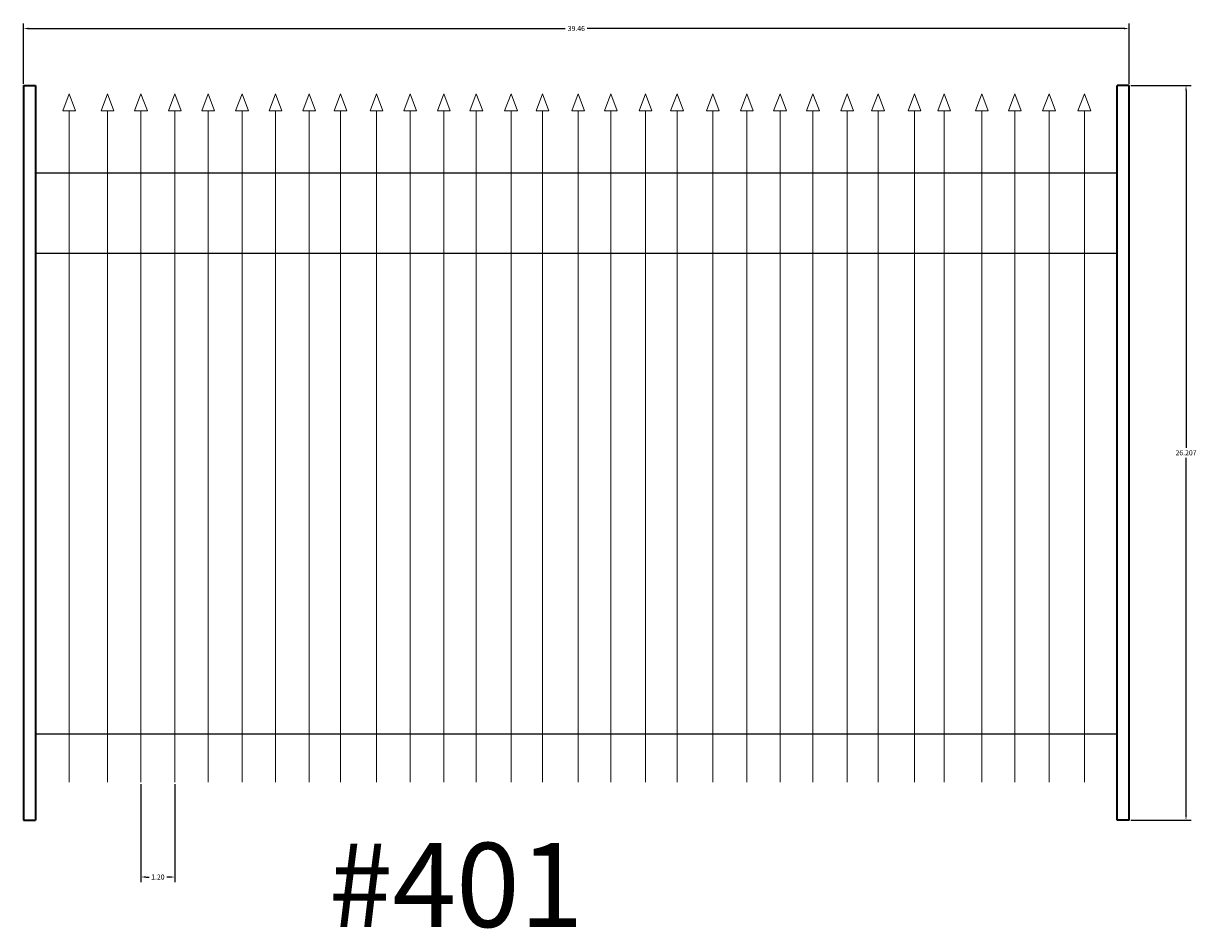
# Model space of a CAD drawing. Units: inches. Extents: x 756 to 915, y 488 to 695.
# Tile 23 of 25: x 866 to 908, y 626 to 659. Entities that reach past the tile are written whole.
import ezdxf

# ---------------------------------------------------------------- set-up
doc = ezdxf.new("R2010")
doc.units = ezdxf.units.IN
doc.header["$MEASUREMENT"] = 0
for name, color, linetype, lineweight in [('L-ANNO-TEXT', 7, 'Continuous', 25), ('L-FENC-PCKT', 7, 'Continuous', 18), ('L-FENC-POST', 7, 'Continuous', 35), ('L-FENC-RAIL', 7, 'Continuous', 25), ('M-DIMS', 2, 'Continuous', 18)]:
    doc.layers.add(name, color=color, linetype=linetype, lineweight=lineweight)
doc.styles.get("Standard").update_dxf_attribs({"font": 'arial.ttf'})
doc.dimstyles.get("Standard").update_dxf_attribs({"dimtxt": 0.18, "dimasz": 0.18, "dimexe": 0.18, "dimexo": 0.0625, "dimgap": 0.09, "dimtad": 0, "dimtih": 1, "dimtoh": 1, "dimdec": 0, "dimzin": 0, "dimdsep": 46, "dimlunit": 3, "dimtxsty": 'Standard', "dimcen": 0.09, "dimadec": 0, "dimazin": 0, "dimtfac": 1, "dimtdec": 0, "dimtofl": 0, "dimtmove": 0, "dimatfit": 3, "dimfxl": 1, "dimtolj": 1, "dimtzin": 0, "dimarcsym": 0})

# ---------------------------------------------------------------- blocks, each defined once
blk = doc.blocks.new('PICKET-SPEAR-EXTENDED')
blk.add_line((0.228, 23.946), (0.228, 0))
blk.add_lwpolyline([(0.228, 23.946), (0, 23.946), (0.228, 24.558), (0.455, 23.946)], close=True)
blk = doc.blocks.new('FENCE-POST-LEFT')
for p, q in [((0, 26.207), (0, 0)), ((0, 26.207), (0.426, 26.207)), ((0.426, 26.207), (0.426, 0)), ((0.426, 26.207), (0.426, 0)), ((0, 0), (0.426, 0))]:
    blk.add_line(p, q)
blk = doc.blocks.new('FENCE-POST-RIGHT')
for p, q in [((0, 26.207), (0, 0)), ((0, 26.207), (0.427, 26.207)), ((0.427, 26.207), (0.427, 0)), ((0, 0), (0.427, 0))]:
    blk.add_line(p, q)
blk = doc.blocks.new('*D41')
at = {"layer": 'Defpoints', "color": 0, "transparency": 16777216}
for p in [(905.412, 658.397), (865.954, 656.367), (905.412, 656.367)]:
    blk.add_point(p, dxfattribs=at)
at = {"layer": 'M-DIMS', "color": 0, "lineweight": -2, "transparency": 16777216}
for p, q in [((865.954, 656.429), (865.954, 658.577)), ((905.412, 656.429), (905.412, 658.577)), ((866.134, 658.397), (885.289, 658.397)), ((905.232, 658.397), (886.076, 658.397))]:
    blk.add_line(p, q, dxfattribs=at)
at = {"layer": 'M-DIMS', "color": 0, "transparency": 16777216}
for points in [[(866.134, 658.427), (866.134, 658.367), (865.954, 658.397)], [(905.232, 658.427), (905.232, 658.367), (905.412, 658.397)]]:
    blk.add_solid(points, dxfattribs=at)
at = {"layer": 'M-DIMS', "color": 0, "transparency": 16777216, "insert": (885.683, 658.397), "char_height": 0.18, "attachment_point": 5}
blk.add_mtext('\\A1;39.46', dxfattribs=at)
blk = doc.blocks.new('*D42')
at = {"layer": 'Defpoints', "color": 0, "transparency": 16777216}
for p in [(905.412, 656.367), (907.442, 656.367), (905.412, 630.16)]:
    blk.add_point(p, dxfattribs=at)
at = {"layer": 'M-DIMS', "color": 0, "lineweight": -2, "transparency": 16777216}
for p, q in [((905.474, 656.367), (907.622, 656.367)), ((907.442, 656.187), (907.442, 643.445)), ((907.442, 630.34), (907.442, 643.081)), ((905.474, 630.16), (907.622, 630.16))]:
    blk.add_line(p, q, dxfattribs=at)
at = {"layer": 'M-DIMS', "color": 0, "transparency": 16777216}
for points in [[(907.412, 656.187), (907.472, 656.187), (907.442, 656.367)], [(907.412, 630.34), (907.472, 630.34), (907.442, 630.16)]]:
    blk.add_solid(points, dxfattribs=at)
at = {"layer": 'M-DIMS', "color": 0, "transparency": 16777216, "insert": (907.442, 643.263), "char_height": 0.18, "attachment_point": 5}
blk.add_mtext('\\A1;26.207', dxfattribs=at)
blk = doc.blocks.new('*D43')
at = {"layer": 'Defpoints', "color": 0, "transparency": 16777216}
for p in [(870.147808, 631.509401), (871.352672, 631.509401), (871.352672, 628.129849)]:
    blk.add_point(p, dxfattribs=at)
at = {"layer": 'M-DIMS', "color": 0, "lineweight": -2, "transparency": 16777216}
for p, q in [((870.147808, 631.446901), (870.147808, 627.949849)), ((871.352672, 631.446901), (871.352672, 627.949849)), ((870.327808, 628.129849), (870.43524, 628.129849)), ((871.172672, 628.129849), (871.06524, 628.129849))]:
    blk.add_line(p, q, dxfattribs=at)
at = {"layer": 'M-DIMS', "color": 0, "transparency": 16777216}
for points in [[(870.327808, 628.159849), (870.327808, 628.099849), (870.147808, 628.129849)], [(871.172672, 628.159849), (871.172672, 628.099849), (871.352672, 628.129849)]]:
    blk.add_solid(points, dxfattribs=at)
at = {"layer": 'M-DIMS', "color": 0, "transparency": 16777216, "insert": (870.75024, 628.129849), "char_height": 0.18, "attachment_point": 5}
blk.add_mtext('\\A1;1.20', dxfattribs=at)

msp = doc.modelspace()

# ---------------------------------------------------------------- linework, layer by layer
at = {"layer": 'L-FENC-RAIL'}
for p, q in [((866.3803, 653.2517), (904.9851, 653.2517)), ((866.3803, 650.3873), (904.9851, 650.3873)), ((866.3803, 633.2415), (904.9851, 633.2415))]:
    msp.add_line(p, q, dxfattribs=at)

# ---------------------------------------------------------------- block references
at = {"layer": 'L-FENC-PCKT'}
for p in [(867.3589, 631.5098), (868.7251, 631.5098), (869.9201, 631.5098), (871.125, 631.5098), (872.3214, 631.5098), (873.5249, 631.5098), (874.7226, 631.5098), (875.9248, 631.5098), (877.0438, 631.5098), (878.3247, 631.5098), (879.525, 631.5098), (880.7247, 631.5098), (881.8862, 631.5098), (883.1246, 631.5098), (884.2474, 631.5098), (885.5245, 631.5098), (886.6887, 631.5098), (887.9244, 631.5098), (889.0499, 631.5098), (890.3243, 631.5098), (891.5394, 631.5098), (892.7242, 631.5098), (893.9006, 631.5098), (895.1241, 631.5098), (896.2218, 631.5098), (897.524, 631.5098), (898.583, 631.5098), (899.9239, 631.5098), (901.1043, 631.5098), (902.3239, 631.5098), (903.5855, 631.5098)]:
    msp.add_blockref('PICKET-SPEAR-EXTENDED', p, dxfattribs=at)
at = {"layer": 'L-FENC-POST'}
msp.add_blockref('FENCE-POST-LEFT', (865.954, 630.1598), dxfattribs=at)
at = {"layer": 'L-FENC-POST', "rotation": 180}
msp.add_blockref('FENCE-POST-RIGHT', (905.4119, 656.3667), dxfattribs=at)

# ---------------------------------------------------------------- texts
at = {"layer": 'L-ANNO-TEXT'}
msp.add_text('#401', height=3, dxfattribs=at).set_placement((876.8488, 626.3457))

# ---------------------------------------------------------------- dimensions: what is measured, and where the dimension line sits
at = {"layer": 'M-DIMS'}
for base, p1, p2, picture, middle in [((905.4118, 658.3967), (865.9536, 656.3667), (905.4118, 656.3667), '*D41', (885.6827, 658.3967)), ((871.3527, 628.1298), (870.1478, 631.5094), (871.3527, 631.5094), '*D43', (870.7502, 628.1298))]:
    dim = msp.add_linear_dim(base=base, p1=p1, p2=p2, dimstyle='Standard', override={"dimdec": 2, "dimlfac": 1, "dimrnd": 0, "dimzin": 0, "dimdsep": 46, "dimlunit": 2}, dxfattribs=at)
    dim.commit()
    dim.dimension.update_dxf_attribs({"geometry": picture, "text_midpoint": middle})
dim = msp.add_linear_dim(base=(907.4418, 656.3667), p1=(905.4118, 630.1598), p2=(905.4118, 656.3667), angle=90, dimstyle='Standard', override={"dimdec": 3, "dimlfac": 1, "dimrnd": 0, "dimzin": 0, "dimdsep": 46, "dimlunit": 2}, dxfattribs=at)
dim.commit()
dim.dimension.update_dxf_attribs({"geometry": '*D42', "text_midpoint": (907.4418, 643.2633)})

doc.saveas('drawing.dxf')
